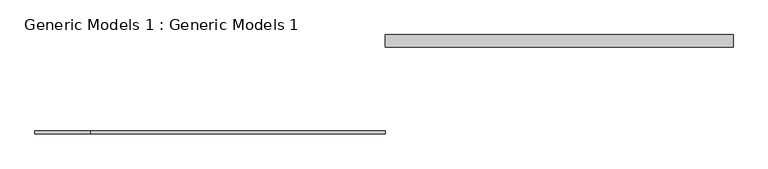
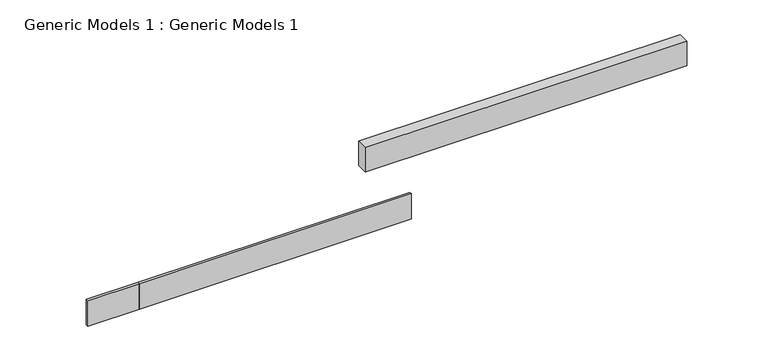
"""IFC4 building model written with IfcOpenShell, lengths in millimetres: proxy geometry, Generic Models 1 : Generic Models 1."""

from ifc_helpers import new_model, si_unit, frame, origin, place, context, project, spatial, polyline, outline, extrude, source, transform, mapped, element, save


def generic_models_1_generic_models_1_5385a8bd(model_context):
    return source(origin(), model_context, "Body", "SweptSolid", [
        extrude(outline(polyline([(-12837.2306534, 2984.1598519), (-13345.2306534, 2984.1598519), (-13345.2306534, 3009.5598519), (-12837.2306534, 3009.5598519), (-12837.2306534, 2984.1598519)])), frame((0.0, 0.0, 8186.2074737), z_axis=(0.0, 0.0, 1.0), x_axis=(1.0, 0.0, 0.0)), (0.0, 0.0, 1.0), 265.6246351),
        extrude(outline(polyline([(-6964.1465329, 3779.5547737), (-10144.8306534, 3779.5547737), (-10144.8306534, 3890.6797737), (-6964.1465329, 3890.6797737), (-6964.1465329, 3779.5547737)])), frame((0.0, 0.0, 8197.9469672), z_axis=(0.0, 0.0, 1.0), x_axis=(1.0, 0.0, 0.0)), (0.0, 0.0, 1.0), 253.8851416),
        extrude(outline(polyline([(-10144.8306534, 2984.1598519), (-12837.2306534, 2984.1598519), (-12837.2306534, 3009.5598519), (-10144.8306534, 3009.5598519), (-10144.8306534, 2984.1598519)])), frame((0.0, 0.0, 8186.2074737), z_axis=(0.0, 0.0, 1.0), x_axis=(1.0, 0.0, 0.0)), (0.0, 0.0, 1.0), 265.6246351),
    ])


if __name__ == "__main__":
    model = new_model("IFC4")
    model_context = context("Model", 3, world=origin())
    ifc_project = project(units=[si_unit("LENGTHUNIT", "METRE", prefix="MILLI")], contexts=[model_context])
    site = spatial("IfcSite", under=ifc_project)
    building = spatial("IfcBuilding", under=site)
    placement = place(None, origin())
    generic_models_1_generic_models_1_shape = generic_models_1_generic_models_1_5385a8bd(model_context)
    element("IfcBuildingElementProxy", 1, Name="Generic Models 1 : Generic Models 1", ObjectType="Generic Models 1 : Generic Models 1", at=placement, inside=building, context=model_context, shape_type="MappedRepresentation", body=[
        mapped(generic_models_1_generic_models_1_shape, transform((0.0, 0.0, 0.0), x_axis=(1.0, 0.0, 0.0), y_axis=(0.0, 1.0, 0.0), z_axis=(0.0, 0.0, 1.0))),
    ])
    save(model, "model.ifc")
